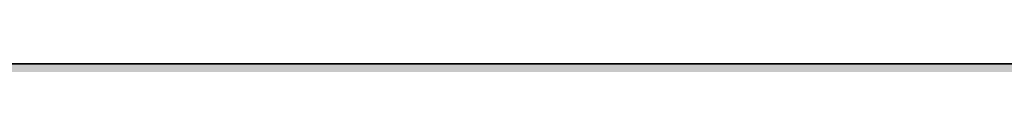
# Model space of a CAD drawing. Units: inches. Extents: x 2091 to 2899, y 967 to 2217.
# Tile 97 of 256: x 2251.8124 to 2252.3817, y 1099.9191 to 1099.9191. Entities that reach past the tile are written whole.
import ezdxf

# ---------------------------------------------------------------- set-up
doc = ezdxf.new("R2010")
doc.units = ezdxf.units.IN
doc.layers.add('A-WALL-PATT', color=141, linetype='Continuous', lineweight=13, true_color=0xadddf7)
doc.layers.add('L-SITE-WALL', color=7, linetype='Continuous', lineweight=35)

msp = doc.modelspace()

# ---------------------------------------------------------------- hatches: boundary and pattern name
at = {"layer": 'A-WALL-PATT'}
h = msp.add_hatch(color=256, dxfattribs=at)
h.dxf.hatch_style = 1
h.paths.add_polyline_path([(2212.1436, 1941.41906), (2387.6436, 1941.41906), (2387.6436, 1824.41906), (2392.1436, 1824.41906), (2392.1436, 1941.41906), (2609.6436, 1941.41906), (2609.6436, 1825.91906), (2614.1436, 1825.91906), (2614.1436, 1941.41906), (2794.1436, 1941.41906), (2794.1436, 1928.76217), (2803.1436, 1928.76217), (2803.1436, 2050.91906), (2203.1436, 2050.91906), (2203.1436, 1900.75786), (2212.1436, 1900.75786)])
h.paths.add_polyline_path([(2212.1436, 1945.91906), (2212.1436, 2041.91906), (2794.1436, 2041.91906), (2794.1436, 1945.91906), (2402.24824, 1945.91906), (2401.10243, 1945.77583), (2398.70243, 1945.77583)], flags=16)
h.paths.add_polyline_path([(2230.22986, 1948.06279), (2227.34986, 1949.50279), (2225.90986, 1951.90279), (2223.98986, 1952.86279), (2223.02986, 1955.26279), (2222.06986, 1959.58279), (2222.06986, 1963.42279), (2223.02986, 1965.66279), (2223.98986, 1965.34279), (2225.58591, 1963.86075), (2226.91153, 1964.95726), (2226.94886, 1965.93879), (2227.77832, 1966.95214), (2228.19992, 1968.8787), (2230.70986, 1964.86279), (2233.58986, 1966.30279), (2233.60731, 1966.33187), (2233.77266, 1964.9382), (2234.6338, 1963.67647), (2235.02986, 1963.90279), (2236.28203, 1965.57236), (2235.98986, 1962.94279), (2237.95451, 1957.54), (2238.38986, 1957.90279), (2239.21586, 1960.30579), (2238.65457, 1966.38496), (2238.69279, 1966.43807), (2238.84058, 1967.49971), (2238.78029, 1967.68749), (2238.88054, 1967.78676), (2238.66686, 1966.25179), (2239.21586, 1960.30579), (2238.38986, 1957.90279), (2236.94986, 1956.70279), (2234.54986, 1949.98279)], flags=0)
h.paths.add_polyline_path([(2278.01197, 1948.06279), (2276.49643, 1947.87335), (2275.84983, 1947.68861), (2274.65197, 1947.10279)], flags=0)
h.paths.add_polyline_path([(2269.85197, 1955.74279), (2268.27618, 1956.62933), (2270.8673, 1956.3484), (2269.37197, 1958.14279), (2268.71496, 1959.19233), (2270.56983, 1958.72861), (2268.58073, 1961.90609), (2270.81197, 1960.89188), (2270.81197, 1963.42279), (2271.39331, 1964.77926), (2270.29176, 1966.1562), (2271.77197, 1965.66279), (2272.14139, 1966.52476), (2273.92983, 1965.92861), (2275.63039, 1968.0543), (2276.33194, 1966.72186), (2276.52043, 1966.95214), (2276.94203, 1968.8787), (2277.73429, 1967.61108), (2278.13989, 1969.46452), (2279.65912, 1967.03374), (2280.41197, 1966.78279), (2280.9493, 1967.58879), (2281.60983, 1967.36861), (2282.13327, 1968.15376), (2282.34924, 1966.33344), (2282.34985, 1966.33259), (2283.40755, 1968.09542), (2283.71263, 1965.52402), (2284.32022, 1964.63379), (2284.51181, 1964.88924), (2284.23497, 1965.70479), (2284.50047, 1967.31896), (2284.90794, 1965.41742), (2285.39631, 1966.06858), (2285.43283, 1966.29061), (2285.47334, 1966.17128), (2286.35392, 1967.34539), (2286.22201, 1966.15817), (2287.66349, 1968.08015), (2287.71397, 1968.44279), (2288.4816, 1969.01668), (2288.57399, 1968.7289), (2288.91746, 1969.06904), (2288.60683, 1966.83761), (2288.92873, 1963.35131), (2288.93497, 1963.35679), (2288.92973, 1963.34042), (2289.01528, 1962.41387), (2290.11122, 1963.87513), (2290.13283, 1963.94261), (2290.21767, 1964.01706), (2290.11122, 1963.87513), (2289.15583, 1960.89161), (2288.59404, 1959.25723), (2288.57197, 1959.10279), (2289.53197, 1960.54279), (2290.01197, 1962.46279), (2290.19184, 1962.64266), (2289.76983, 1959.68861), (2286.88983, 1957.28861), (2284.48983, 1950.56861), (2283.31466, 1950.04631), (2283.29197, 1949.98279), (2280.29006, 1948.64861), (2281.12983, 1948.64861), (2282.56983, 1948.16861), (2283.20473, 1948.06279), (2278.97197, 1948.06279), (2276.09197, 1949.50279), (2274.65197, 1951.90279), (2272.73197, 1952.86279)], flags=0)
h.paths.add_polyline_path([(2271.15887, 1958.02177), (2272.96983, 1955.84861), (2272.00983, 1960.16861), (2272.00983, 1964.00861), (2272.62443, 1965.44266), (2274.32802, 1963.86075), (2275.65365, 1964.95726), (2275.63774, 1964.53909), (2277.41223, 1966.00689), (2277.03297, 1965.15679), (2276.82992, 1964.9756), (2276.76601, 1963.29501), (2277.44964, 1962.66022), (2279.45197, 1964.86279), (2282.33197, 1966.30279), (2283.52983, 1966.88861), (2283.29451, 1966.77095), (2283.91299, 1963.8847), (2284.89925, 1964.44827), (2284.73197, 1962.94279), (2286.69662, 1957.54), (2287.13197, 1957.90279), (2287.54191, 1959.09539), (2287.7794, 1958.44231), (2285.68274, 1956.6951), (2285.8765, 1959.79534), (2284.73197, 1962.94279), (2284.89925, 1964.44827), (2283.91299, 1963.8847), (2284.22383, 1962.43412), (2283.42436, 1963.60548), (2281.60983, 1962.56861), (2281.12983, 1960.16861), (2282.08983, 1956.32861), (2283.04983, 1952.96861), (2282.56983, 1950.56861), (2280.16983, 1948.64861), (2279.88332, 1948.79187), (2278.97197, 1948.06279), (2278.97197, 1949.02279), (2278.67231, 1949.39737), (2277.28983, 1950.08861), (2275.84983, 1952.48861), (2273.92983, 1953.44861), (2272.48983, 1954.88861), (2271.92165, 1954.88861), (2271.77197, 1955.26279)], flags=0)
h.paths.add_polyline_path([(2311.99415, 1955.74279), (2312.06272, 1955.67422), (2312.0551, 1955.7085)], flags=0)
h.paths.add_polyline_path([(2331.95615, 1963.95179), (2333.39615, 1965.39179), (2331.07715, 1963.35679), (2330.9986, 1963.11152)], flags=0)
h.paths.add_polyline_path([(2310.55415, 1954.30279), (2307.03981, 1956.27994), (2310.7629, 1955.87628), (2312.47415, 1953.82279), (2313.43415, 1951.42279), (2315.35415, 1950.46279), (2316.79415, 1948.06279), (2317.46615, 1947.72679), (2319.36869, 1947.96461), (2317.75415, 1949.98279), (2317.56953, 1950.61048), (2316.79415, 1951.90279), (2314.87415, 1952.86279), (2313.91415, 1955.26279), (2311.51415, 1958.14279), (2309.37549, 1961.55917), (2311.51415, 1960.33708), (2311.51415, 1961.98279), (2310.60467, 1963.11963), (2311.72661, 1962.47853), (2312.41833, 1964.09256), (2312.25596, 1964.29552), (2313.19415, 1963.98279), (2313.91415, 1965.66279), (2314.64678, 1965.41858), (2315.35415, 1966.30279), (2316.79415, 1967.74279), (2316.15744, 1966.9469), (2317.03411, 1965.28186), (2317.2226, 1965.51214), (2317.77705, 1968.04577), (2318.47411, 1966.72186), (2318.6626, 1966.95214), (2319.0842, 1968.8787), (2321.20705, 1965.48215), (2322.16142, 1966.9137), (2322.55415, 1966.78279), (2322.78599, 1967.13056), (2322.88165, 1966.32429), (2323.31204, 1965.72174), (2323.65129, 1965.89136), (2324.3965, 1967.13338), (2324.65694, 1964.9382), (2324.97199, 1964.47661), (2325.38728, 1967.0015), (2325.94081, 1964.41835), (2327.22893, 1966.13584), (2327.16632, 1965.57236), (2328.05914, 1966.76278), (2328.22458, 1966.24749), (2329.66797, 1967.67691), (2329.66458, 1967.68749), (2329.76482, 1967.78676), (2329.55115, 1966.25179), (2330.10015, 1960.30579), (2329.33281, 1958.07347), (2329.31306, 1957.93523), (2329.63415, 1958.20279), (2330.23415, 1959.10279), (2330.71415, 1961.02279), (2331.03415, 1961.34279), (2330.71415, 1959.10279), (2329.63415, 1958.20279), (2329.27415, 1957.66279), (2327.71211, 1956.3611), (2325.43415, 1949.98279), (2324.33377, 1949.49374), (2323.99415, 1948.54279), (2319.67415, 1946.62279), (2316.79415, 1948.06279), (2315.35415, 1950.46279), (2313.43415, 1951.42279)], flags=0)
h.paths.add_polyline_path([(2321.33568, 1947.95202), (2321.11415, 1948.06279), (2321.11415, 1949.02279), (2319.19415, 1951.42279), (2316.79415, 1959.58279), (2316.66324, 1959.58279), (2315.35415, 1958.14279), (2314.39415, 1958.14279), (2313.1483, 1958.70908), (2312.95415, 1959.58279), (2312.95415, 1960.89188), (2315.83415, 1959.58279), (2316.66324, 1959.58279), (2317.31471, 1960.29941), (2315.0302, 1962.42075), (2316.35582, 1963.51726), (2316.37234, 1963.95162), (2316.4702, 1963.86075), (2317.79582, 1964.95726), (2317.75522, 1963.88969), (2319.17515, 1965.15679), (2319.49841, 1965.88137), (2321.11415, 1965.34279), (2323.23589, 1962.37236), (2325.68635, 1963.77262), (2325.54279, 1962.48058), (2325.19878, 1963.49401), (2324.47851, 1963.08243), (2324.92601, 1960.99412), (2324.07809, 1962.23647), (2322.41479, 1961.28602), (2322.07415, 1959.58279), (2323.03415, 1955.74279), (2323.99415, 1952.38279), (2323.51415, 1949.98279), (2322.14272, 1948.88565), (2322.07415, 1948.54279)], flags=0)
h.paths.add_polyline_path([(2320.20748, 1963.33746), (2320.15415, 1963.42279), (2320.39415, 1963.54279)], flags=0)
h.paths.add_polyline_path([(2353.85053, 1965.8105), (2354.03053, 1965.7505), (2354.33053, 1966.4505), (2354.33053, 1966.9305)], flags=0)
h.paths.add_polyline_path([(2359.02058, 1969.02641), (2359.09838, 1968.90193), (2359.23353, 1969.5195), (2359.23353, 1969.9995)], flags=0)
h.paths.add_polyline_path([(2358.25669, 1966.68167), (2357.9836, 1966.34803), (2358.21127, 1966.14617), (2358.41049, 1966.38957)], flags=0)
h.paths.add_polyline_path([(2357.76847, 1966.05878), (2357.7322, 1965.10497), (2357.75105, 1965.12056), (2357.76953, 1965.6065), (2357.76953, 1966.05784)], flags=0)
h.paths.add_polyline_path([(2359.11153, 1965.3045), (2359.11153, 1964.8245), (2359.84453, 1966.4675), (2359.84453, 1966.9475)], flags=0)
h.paths.add_polyline_path([(2360.22368, 1966.62145), (2360.69853, 1969.3625), (2360.69853, 1969.8425), (2360.21053, 1967.0255), (2360.21053, 1966.6425)], flags=0)
h.paths.add_polyline_path([(2363.45053, 1967.8905), (2363.45053, 1968.3705), (2362.49053, 1966.9305), (2362.65604, 1966.69878)], flags=0)
h.paths.add_polyline_path([(2364.47552, 1966.07883), (2365.85053, 1968.3705), (2365.85053, 1968.8505), (2364.42798, 1966.47958)], flags=0)
h.paths.add_polyline_path([(2366.31353, 1965.8525), (2366.36671, 1965.69583), (2366.80253, 1968.3455), (2366.80253, 1968.8255)], flags=0)
h.paths.add_polyline_path([(2367.16531, 1965.80354), (2367.29053, 1966.9305), (2367.29053, 1967.4105), (2367.1027, 1965.72007)], flags=0)
h.paths.add_polyline_path([(2370.03653, 1959.9735), (2371.01353, 1963.0245), (2371.01353, 1963.5045), (2370.03653, 1960.4535)], flags=0)
h.paths.add_polyline_path([(2371.61053, 1960.2105), (2372.57053, 1961.6505), (2372.57053, 1962.1305), (2371.80253, 1960.9785)], flags=0)
h.paths.add_polyline_path([(2350.87367, 1956.00509), (2351.93053, 1955.8905), (2354.49053, 1953.3305), (2353.85053, 1954.9305), (2351.45053, 1957.8105), (2347.93553, 1963.4255), (2347.93553, 1963.9055), (2351.45053, 1958.2905), (2353.70507, 1955.58505), (2352.89053, 1959.2505), (2352.89053, 1959.7305), (2352.89053, 1961.92479), (2356.73053, 1959.7305), (2358.45447, 1961.62684), (2354.81053, 1965.0105), (2355.03086, 1965.28591), (2358.69109, 1961.88712), (2361.53053, 1965.0105), (2364.3765, 1966.43348), (2364.52439, 1965.18691), (2365.45447, 1963.82418), (2365.88107, 1964.06795), (2365.37053, 1966.4505), (2365.37053, 1966.9305), (2366.81053, 1960.2105), (2366.81053, 1959.7305), (2366.38871, 1952.98141), (2367.77053, 1956.8505), (2368.64123, 1957.57608), (2366.81053, 1962.6105), (2366.81053, 1963.0905), (2368.77518, 1957.68771), (2369.21053, 1958.0505), (2370.00159, 1960.35187), (2369.47523, 1966.05267), (2369.51346, 1966.10578), (2369.51417, 1966.11091), (2369.47523, 1966.53267), (2369.51346, 1966.58578), (2369.61463, 1967.31259), (2369.18253, 1968.6585), (2369.18253, 1969.1385), (2369.60096, 1967.83519), (2369.7012, 1967.93447), (2369.71795, 1968.05474), (2370.14518, 1968.37414), (2369.77871, 1968.01122), (2369.7012, 1967.45447), (2370.46816, 1968.214), (2369.67494, 1967.26577), (2369.51417, 1966.11091), (2370.03653, 1960.4535), (2370.03653, 1959.9735), (2369.44176, 1958.24319), (2370.65053, 1959.2505), (2371.04582, 1962.01756), (2371.13053, 1962.1305), (2370.65053, 1958.7705), (2367.77053, 1956.3705), (2365.37053, 1949.6505), (2362.0791, 1948.18764), (2363.45053, 1947.7305), (2361.05053, 1947.7305), (2360.09053, 1947.7305), (2357.10386, 1947.35717), (2360.09053, 1948.2105), (2358.17053, 1949.1705), (2356.73053, 1951.5705), (2354.81053, 1952.5305), (2351.93053, 1955.4105)], flags=0)
h.paths.add_polyline_path([(2361.05053, 1948.6905), (2359.13053, 1951.0905), (2356.73053, 1959.2505), (2355.77053, 1959.2505), (2352.89053, 1960.55959), (2352.89053, 1961.44479), (2355.89053, 1959.7305), (2356.73053, 1959.7305), (2356.83719, 1959.36783), (2361.53053, 1964.5305), (2363.24842, 1965.38945), (2364.92531, 1963.0418), (2362.49053, 1961.6505), (2362.06386, 1959.51717), (2362.97053, 1955.8905), (2363.93053, 1952.5305), (2363.93053, 1952.0505), (2363.45053, 1949.6505), (2361.05053, 1947.7305)], flags=0)
h.paths.add_polyline_path([(2359.13053, 1951.5705), (2359.29053, 1951.3705), (2361.05053, 1954.4505), (2361.05053, 1954.9305)], flags=0)
h.paths.add_polyline_path([(2357.21953, 1966.5455), (2356.79253, 1968.8145), (2356.79253, 1969.2945), (2357.21953, 1967.0255)], flags=0)
h.paths.add_polyline_path([(2361.05053, 1954.4505), (2361.53053, 1958.7705), (2361.53053, 1959.2505), (2361.05053, 1954.9305)], flags=0)
h.paths.add_polyline_path([(2402.54829, 1948.48608), (2402.30243, 1948.41583), (2402.59043, 1948.41583)], flags=0)
h.paths.add_polyline_path([(2394.14243, 1956.09583), (2395.68505, 1954.55321), (2396.7205, 1953.97068), (2396.06243, 1955.61583), (2395.24138, 1956.6011), (2395.8789, 1956.44171), (2395.10243, 1959.93583), (2395.10243, 1963.77583), (2396.06243, 1966.01583), (2397.02243, 1965.69583), (2398.61848, 1964.21379), (2399.94411, 1965.3103), (2399.98143, 1966.29183), (2400.81089, 1967.30518), (2401.23249, 1969.23174), (2403.53795, 1965.54301), (2403.94198, 1967.38932), (2404.70243, 1967.13583), (2405.46033, 1966.07478), (2406.62243, 1966.65583), (2406.63988, 1966.68491), (2406.80523, 1965.29124), (2406.92569, 1965.11475), (2407.34243, 1964.97583), (2407.87433, 1965.77367), (2408.1691, 1964.39805), (2409.31461, 1965.9254), (2409.21746, 1965.05105), (2409.44523, 1963.13124), (2410.30637, 1961.86951), (2410.70243, 1962.09583), (2411.44227, 1963.08228), (2411.16543, 1963.89783), (2411.61643, 1966.63976), (2411.72536, 1966.79111), (2411.87315, 1967.85275), (2411.81286, 1968.04053), (2411.91311, 1968.1398), (2411.69943, 1966.60483), (2412.24843, 1960.65883), (2413.22543, 1963.70983), (2414.3779, 1964.72116), (2414.51315, 1965.69275), (2414.45286, 1965.88053), (2414.55311, 1965.9798), (2414.3779, 1964.72116), (2414.51982, 1964.8457), (2414.36536, 1964.63111), (2414.33943, 1964.44483), (2414.88843, 1958.49883), (2414.06243, 1956.09583), (2412.62243, 1954.89583), (2410.17137, 1948.03285), (2410.01672, 1948.0844), (2405.90243, 1946.25583), (2405.90243, 1947.21583), (2405.20425, 1948.08856), (2404.22243, 1948.41583), (2403.26243, 1948.41583), (2400.38243, 1949.85583), (2399.66243, 1951.05583), (2397.98243, 1952.73583), (2397.02243, 1953.21583), (2395.68505, 1954.55321), (2392.65678, 1956.25691)], flags=0)
h.paths.add_polyline_path([(2409.08565, 1964.40744), (2409.13036, 1964.27572), (2409.26243, 1964.49583)], flags=0)
h.paths.add_polyline_path([(2397.74243, 1961.61583), (2398.70243, 1963.85583), (2399.66243, 1963.53583), (2401.42656, 1965.74099), (2401.79142, 1966.5588), (2402.07143, 1965.07083), (2402.83551, 1964.39337), (2403.2624, 1964.9149), (2403.33812, 1964.77109), (2402.61552, 1963.97622), (2402.49861, 1960.90224), (2403.543, 1959.93245), (2404.4132, 1960.88968), (2404.70243, 1962.33583), (2407.91635, 1964.17235), (2409.52021, 1961.92694), (2410.98708, 1957.89304), (2411.42243, 1958.25583), (2412.04796, 1960.07562), (2412.41034, 1959.07909), (2411.67562, 1958.46682), (2411.66243, 1958.25583), (2411.62607, 1958.42553), (2409.98243, 1957.05583), (2407.58243, 1950.33583), (2403.26243, 1948.41583), (2403.26243, 1949.37583), (2401.34243, 1951.77583), (2399.41651, 1958.32398), (2397.74243, 1959.08492), (2397.74243, 1959.97012), (2397.10243, 1960.33583), (2397.74243, 1960.04492)], flags=0)
h.paths.add_polyline_path([(2405.90243, 1952.97583), (2405.95043, 1953.40783), (2406.01672, 1953.17583)], flags=0)
h.paths.add_polyline_path([(2449.81778, 1967.11401), (2449.75232, 1967.13583), (2449.7937, 1967.0779)], flags=0)
h.paths.add_polyline_path([(2451.6977, 1966.61812), (2451.74089, 1966.69012), (2451.69205, 1966.6657)], flags=0)
h.paths.add_polyline_path([(2454.34363, 1965.73757), (2455.75232, 1967.61583), (2455.99232, 1968.09583), (2454.3645, 1965.9254)], flags=0)
h.paths.add_polyline_path([(2457.54732, 1968.86383), (2457.78732, 1969.34383), (2457.05432, 1968.79583), (2457.00762, 1968.46034)], flags=0)
h.paths.add_polyline_path([(2456.92178, 1967.85666), (2456.80224, 1968.22902), (2456.723, 1967.6598)], flags=0)
h.paths.add_polyline_path([(2457.30232, 1967.37683), (2457.54232, 1967.85683), (2456.81032, 1966.83983), (2456.74052, 1966.70022), (2456.74902, 1966.60811)], flags=0)
h.paths.add_polyline_path([(2458.27532, 1963.70983), (2458.15534, 1963.33515), (2460.35432, 1965.26483), (2460.59432, 1965.74483)], flags=0)
h.paths.add_polyline_path([(2458.39232, 1962.81583), (2458.36409, 1962.61819), (2459.59232, 1964.25583), (2459.83232, 1964.73583)], flags=0)
h.paths.add_polyline_path([(2459.35232, 1962.81583), (2459.27232, 1962.49583), (2460.07232, 1963.29583), (2460.31232, 1963.77583)], flags=0)
h.paths.add_polyline_path([(2458.68032, 1960.60783), (2458.63232, 1960.41583), (2459.59232, 1961.85583), (2459.83232, 1962.33583)], flags=0)
h.paths.add_polyline_path([(2437.83817, 1956.24265), (2439.19232, 1956.09583), (2441.35232, 1953.93583), (2440.87232, 1955.13583), (2438.47232, 1958.01583), (2438.07156, 1958.65602), (2438.71232, 1958.49583), (2440.6396, 1956.18311), (2439.91232, 1959.45583), (2439.91232, 1963.29583), (2441.35232, 1966.65583), (2441.59232, 1967.13583), (2441.11232, 1966.01583), (2442.07232, 1965.69583), (2443.98899, 1968.09167), (2444.24132, 1966.75083), (2444.9168, 1966.15192), (2445.67657, 1967.08014), (2446.25532, 1969.72483), (2446.49532, 1970.20483), (2446.28238, 1969.23174), (2447.36267, 1967.50327), (2447.72032, 1969.56783), (2447.96032, 1970.04783), (2447.48548, 1967.30678), (2448.79232, 1965.21583), (2448.47232, 1964.86383), (2448.55232, 1964.73583), (2451.45205, 1966.1857), (2451.61512, 1964.81124), (2452.30792, 1963.79617), (2453.23451, 1964.32565), (2454.07232, 1960.41583), (2453.62869, 1953.31765), (2454.79232, 1956.57583), (2455.03232, 1957.05583), (2455.71884, 1957.62793), (2453.83232, 1962.81583), (2453.94097, 1963.79362), (2453.33532, 1965.57783), (2453.82432, 1968.55083), (2454.06432, 1969.03083), (2453.57532, 1966.05783), (2454.04033, 1964.68792), (2453.83232, 1962.81583), (2455.71884, 1957.62793), (2456.36721, 1958.16824), (2457.05832, 1960.17883), (2457.29832, 1960.65883), (2456.47232, 1958.25583), (2457.71773, 1959.29367), (2457.67232, 1958.97583), (2454.88995, 1956.65719), (2453.61414, 1953.08492), (2453.59232, 1952.73583), (2453.35232, 1952.25583), (2453.3596, 1952.3722), (2452.63232, 1950.33583), (2452.39232, 1949.85583), (2449.20375, 1948.43869), (2450.71232, 1947.93583), (2448.07232, 1947.93583), (2447.11232, 1947.93583), (2444.55232, 1947.61583), (2447.1996, 1948.3722), (2445.19232, 1949.37583), (2443.75232, 1951.77583), (2441.83232, 1952.73583), (2438.95232, 1955.61583)], flags=0)
h.paths.add_polyline_path([(2443.99232, 1959.93583), (2444.04032, 1959.77263), (2444.12155, 1959.86199)], flags=0)
h.paths.add_polyline_path([(2442.91232, 1959.93583), (2443.03232, 1959.93583), (2442.44566, 1960.2025)], flags=0)
h.paths.add_polyline_path([(2444.98294, 1965.01968), (2445.27932, 1965.26483), (2445.51932, 1965.74483), (2444.994, 1965.3103)], flags=0)
h.paths.add_polyline_path([(2446.13332, 1965.02983), (2446.33037, 1965.4715), (2444.97032, 1964.25783), (2444.73032, 1963.77783)], flags=0)
h.paths.add_polyline_path([(2442.79232, 1959.45583), (2443.75232, 1959.45583), (2446.15232, 1951.29583), (2446.41232, 1951.75083), (2446.39232, 1951.77583), (2448.0806, 1954.73032), (2448.55232, 1958.97583), (2441.83232, 1965.21583), (2442.15495, 1965.61911), (2448.79232, 1959.45583), (2448.31232, 1955.13583), (2448.07232, 1954.65583), (2446.41232, 1951.75083), (2448.31232, 1949.37583), (2448.31232, 1948.41583), (2450.54089, 1950.19869), (2450.95232, 1952.25583), (2449.99232, 1955.61583), (2449.03232, 1959.45583), (2449.51232, 1961.85583), (2449.75232, 1962.33583), (2449.6749, 1961.94874), (2452.99451, 1963.84565), (2453.06441, 1963.51941), (2452.88461, 1963.78285), (2449.6749, 1961.94874), (2449.27232, 1959.93583), (2450.23232, 1956.09583), (2451.19232, 1952.73583), (2450.71232, 1950.33583), (2450.47232, 1949.85583), (2448.07232, 1947.93583), (2448.07232, 1948.53583), (2445.43232, 1949.85583), (2443.99232, 1952.25583), (2442.07232, 1953.21583), (2441.11232, 1955.61583), (2440.15232, 1959.93583), (2440.15232, 1960.65583)], flags=0)
h.paths.add_polyline_path([(2456.69232, 1966.98583), (2457.60832, 1968.08083), (2457.84832, 1968.56083), (2456.93232, 1967.46583)], flags=0)
h.paths.add_polyline_path([(2489.89657, 1966.58024), (2489.94295, 1966.18935), (2490.74749, 1967.53025), (2491.31912, 1968.95116)], flags=0)
h.paths.add_polyline_path([(2473.56247, 1956.40713), (2477.13998, 1956.01926), (2476.95533, 1956.24083), (2475.10805, 1957.28011), (2476.34749, 1956.97025), (2475.1869, 1958.82422), (2476.91912, 1958.39116), (2475.41164, 1960.79927), (2477.78749, 1959.71934), (2477.78749, 1962.25025), (2477.6374, 1962.43786), (2477.82255, 1962.33206), (2478.35912, 1963.58406), (2478.35912, 1963.67116), (2477.32435, 1964.96463), (2478.71483, 1964.50114), (2479.31912, 1965.91116), (2480.27912, 1965.59116), (2481.78397, 1967.47221), (2482.11649, 1965.70525), (2482.88056, 1965.02778), (2483.20931, 1965.42941), (2483.22017, 1965.71509), (2483.07594, 1965.98902), (2483.71176, 1966.76581), (2484.13049, 1968.67925), (2484.70212, 1970.10016), (2484.48918, 1969.12707), (2486.5029, 1965.90511), (2487.38749, 1965.61025), (2488.15342, 1966.75914), (2488.71702, 1965.97011), (2489.20009, 1966.21164), (2489.33067, 1965.11099), (2490.3939, 1963.62246), (2490.66077, 1963.77496), (2490.49391, 1964.55364), (2490.92306, 1963.92484), (2491.31912, 1964.15116), (2491.33339, 1964.17018), (2491.21049, 1964.53225), (2491.28176, 1964.96554), (2491.42579, 1964.29338), (2494.07648, 1967.82763), (2494.49792, 1966.51494), (2494.59817, 1966.61422), (2494.68949, 1967.27025), (2495.10675, 1967.5822), (2495.12984, 1967.74807), (2495.06955, 1967.93585), (2495.1698, 1968.03513), (2495.03178, 1967.04363), (2495.75382, 1967.75868), (2494.98205, 1966.68644), (2494.95612, 1966.50016), (2495.47902, 1960.83685), (2495.91049, 1962.18425), (2496.48212, 1963.60516), (2496.07269, 1962.32659), (2496.7689, 1962.93754), (2496.59912, 1962.71116), (2496.11912, 1959.35116), (2496.73287, 1960.27179), (2496.98749, 1961.29025), (2497.55912, 1962.71116), (2497.07912, 1960.79116), (2496.50749, 1959.37025), (2495.54749, 1957.93025), (2492.75884, 1955.60638), (2490.83912, 1950.23116), (2490.26749, 1948.81025), (2485.94749, 1946.89025), (2483.06749, 1948.33025), (2481.62749, 1950.73025), (2479.70749, 1951.69025), (2476.82749, 1954.57025)], flags=0)
h.paths.add_polyline_path([(2485.57697, 1948.31339), (2485.55912, 1948.31116), (2485.57876, 1948.31116)], flags=0)
h.paths.add_polyline_path([(2478.64506, 1954.55116), (2478.10904, 1956.96326), (2479.31912, 1955.51116), (2480.27912, 1953.11116), (2482.19912, 1952.15116), (2483.63912, 1949.75116), (2486.51912, 1948.31116), (2486.51912, 1949.27116), (2484.73931, 1951.49593), (2484.02749, 1950.25025), (2481.62749, 1958.41025), (2482.37515, 1959.23267), (2482.19912, 1959.83116), (2483.19757, 1960.92946), (2479.70749, 1964.17025), (2480.60336, 1965.29008), (2481.87517, 1964.10911), (2482.66639, 1964.76358), (2482.61536, 1963.4218), (2482.9892, 1963.07466), (2484.00849, 1963.98425), (2484.68361, 1965.49751), (2484.58012, 1965.40516), (2485.35727, 1967.14711), (2485.12065, 1965.7812), (2486.42749, 1963.69025), (2488.14538, 1964.5492), (2489.82227, 1962.20155), (2490.74749, 1962.73025), (2491.99966, 1964.39981), (2492.07605, 1965.08726), (2492.21289, 1964.68412), (2492.48537, 1965.04743), (2492.27912, 1963.19116), (2494.24377, 1957.78837), (2494.5625, 1958.05398), (2494.93349, 1959.13325), (2495.50512, 1960.55416), (2494.67912, 1958.15116), (2494.10749, 1956.73025), (2494.5625, 1958.05398), (2493.40854, 1957.09235), (2491.70749, 1961.77025), (2491.99966, 1964.39981), (2490.74749, 1962.73025), (2487.71203, 1960.9957), (2487.47912, 1959.83116), (2488.43912, 1955.99116), (2489.39912, 1952.63116), (2488.91912, 1950.23116), (2488.57692, 1949.9574), (2488.34749, 1948.81025), (2487.65172, 1948.25363), (2487.47912, 1948.31116), (2486.51912, 1948.31116), (2483.63912, 1949.75116), (2482.19912, 1952.15116), (2480.27912, 1953.11116), (2478.83912, 1954.55116)], flags=0)
h.paths.add_polyline_path([(2526.64825, 1966.98752), (2526.51734, 1967.03116), (2526.6001, 1966.9153)], flags=0)
h.paths.add_polyline_path([(2528.47064, 1966.44666), (2528.57449, 1966.61973), (2528.45707, 1966.56102)], flags=0)
h.paths.add_polyline_path([(2534.13334, 1967.49616), (2534.15669, 1967.54285), (2534.05984, 1967.4083)], flags=0)
h.paths.add_polyline_path([(2536.16192, 1964.0506), (2535.15734, 1962.71116), (2535.10087, 1962.31587), (2536.11734, 1963.67116), (2536.42053, 1964.27754)], flags=0)
h.paths.add_polyline_path([(2535.15734, 1959.83116), (2536.11734, 1961.27116), (2536.59734, 1962.23116), (2535.25334, 1960.21516)], flags=0)
h.paths.add_polyline_path([(2513.24904, 1956.2848), (2516.22118, 1955.96256), (2514.99734, 1957.43116), (2514.19582, 1958.71154), (2515.47734, 1958.39116), (2516.93189, 1956.64571), (2516.43734, 1958.87116), (2516.43734, 1962.71116), (2516.87269, 1963.72697), (2515.34643, 1965.6348), (2517.39734, 1964.95116), (2517.87734, 1966.07116), (2518.35734, 1967.03116), (2517.87734, 1965.91116), (2518.83734, 1965.59116), (2520.48659, 1967.65272), (2520.76634, 1966.16616), (2521.53042, 1965.48869), (2521.78144, 1965.79537), (2521.80091, 1966.30727), (2521.4778, 1966.92094), (2521.24634, 1967.12616), (2521.1777, 1967.49091), (2521.4778, 1966.92094), (2522.01042, 1966.44869), (2522.25739, 1966.75042), (2522.78034, 1969.14016), (2523.26034, 1970.10016), (2523.0474, 1969.12707), (2524.67313, 1966.5259), (2526.03734, 1966.07116), (2526.79524, 1965.01011), (2527.97707, 1965.60102), (2528.14014, 1964.22657), (2528.66459, 1963.45816), (2529.38862, 1963.87189), (2529.32967, 1964.14699), (2529.48128, 1963.92484), (2529.87734, 1964.15116), (2529.98401, 1964.29338), (2529.78905, 1965.20318), (2530.0624, 1964.3979), (2532.80248, 1968.05135), (2533.14777, 1966.97585), (2533.24802, 1967.07513), (2533.33934, 1967.73116), (2533.67285, 1967.98049), (2533.72802, 1968.03513), (2533.51434, 1966.50016), (2534.02472, 1960.9725), (2534.56034, 1962.64516), (2535.04034, 1963.60516), (2534.06334, 1960.55416), (2533.23734, 1958.15116), (2534.28815, 1959.02684), (2534.19734, 1958.39116), (2531.5126, 1956.15387), (2529.39734, 1950.23116), (2528.91734, 1949.27116), (2526.44877, 1948.17402), (2527.47734, 1947.83116), (2530.35734, 1947.35116), (2524.59734, 1947.35116), (2521.71734, 1948.79116), (2520.27734, 1951.19116), (2518.35734, 1952.15116), (2515.47734, 1955.03116)], flags=0)
h.paths.add_polyline_path([(2523.93476, 1967.19031), (2523.61951, 1966.48369), (2523.7705, 1966.24211)], flags=0)
h.paths.add_polyline_path([(2518.83734, 1953.11116), (2517.87734, 1955.51116), (2516.88498, 1959.97678), (2516.91734, 1959.96207), (2516.91734, 1962.02545), (2520.75734, 1959.83116), (2522.02495, 1961.22553), (2518.35734, 1964.63116), (2519.00259, 1965.43772), (2520.43339, 1964.10911), (2521.30112, 1964.82687), (2521.24516, 1963.35533), (2525.63831, 1959.27598), (2526.03734, 1961.27116), (2529.39734, 1963.19116), (2530.64952, 1964.86073), (2530.66472, 1964.99755), (2530.69196, 1964.91731), (2531.08778, 1965.44507), (2530.94599, 1964.16894), (2530.69196, 1964.91731), (2529.39734, 1963.19116), (2526.3625, 1961.45697), (2526.03734, 1959.83116), (2526.99734, 1955.99116), (2527.95734, 1952.63116), (2527.47734, 1950.23116), (2527.13449, 1949.95687), (2526.97393, 1949.15409), (2526.69734, 1949.03116), (2524.59734, 1947.35116), (2524.59734, 1948.31116), (2524.27734, 1948.71116), (2522.19734, 1949.75116), (2520.75734, 1952.15116)], flags=0)
h.paths.add_polyline_path([(2520.27734, 1958.87116), (2520.85334, 1959.50476), (2523.15734, 1951.67116), (2524.61389, 1954.22013), (2524.59734, 1954.07116), (2522.67734, 1950.71116)], flags=0)
h.paths.add_polyline_path([(2559.37091, 1966.31116), (2559.39841, 1966.32491), (2559.40194, 1966.3453)], flags=0)
h.paths.add_polyline_path([(2549.77091, 1957.19116), (2552.65091, 1954.31116), (2552.13399, 1955.60347), (2550.61091, 1957.43116), (2547.09591, 1963.04616), (2545.77591, 1965.20616), (2549.29091, 1959.59116), (2551.69091, 1956.71116), (2550.79293, 1960.75206), (2550.73091, 1960.78025), (2550.73091, 1964.87116), (2551.69091, 1967.11116), (2552.65091, 1966.79116), (2554.24696, 1965.30911), (2555.03425, 1965.96034), (2555.58167, 1966.64461), (2555.60991, 1967.38716), (2556.43937, 1968.40051), (2556.86097, 1970.32707), (2559.37091, 1966.31116), (2560.69091, 1964.15116), (2562.40881, 1965.01011), (2561.65091, 1966.07116), (2560.33091, 1968.23116), (2561.7585, 1966.23254), (2562.34721, 1967.11561), (2562.43371, 1966.38657), (2563.1278, 1965.3696), (2563.57091, 1965.59116), (2563.58836, 1965.62024), (2563.36254, 1967.52354), (2563.72249, 1965.84379), (2565.06, 1968.07298), (2564.73286, 1965.12872), (2565.11758, 1963.33338), (2567.44462, 1966.43611), (2567.31561, 1967.83333), (2567.35384, 1967.88644), (2567.50163, 1968.94807), (2567.44134, 1969.13585), (2567.54159, 1969.23513), (2567.32791, 1967.70016), (2567.87691, 1961.75416), (2568.74669, 1964.47033), (2568.63561, 1965.67333), (2568.67384, 1965.72644), (2568.82163, 1966.78807), (2568.76134, 1966.97585), (2568.86159, 1967.07513), (2568.64791, 1965.54016), (2568.72613, 1964.69303), (2568.85391, 1964.80516), (2568.74669, 1964.47033), (2568.81724, 1963.70626), (2568.97091, 1963.91116), (2568.86607, 1963.17731), (2569.19691, 1959.59416), (2568.37091, 1957.19116), (2566.93091, 1955.99116), (2564.62027, 1949.52137), (2564.65091, 1949.51116), (2564.61662, 1949.51116), (2564.53091, 1949.27116), (2560.21091, 1947.35116), (2557.33091, 1948.79116), (2556.0452, 1950.93402), (2556.01091, 1950.95116), (2555.85662, 1951.2083), (2553.97091, 1952.15116), (2551.09091, 1955.03116), (2546.65014, 1957.52951)], flags=0)
h.paths.add_polyline_path([(2567.02579, 1959.33023), (2567.03501, 1959.30489), (2567.05091, 1959.35116)], flags=0)
h.paths.add_polyline_path([(2551.96829, 1962.51837), (2553.01091, 1964.95116), (2553.97091, 1964.63116), (2555.56696, 1963.14911), (2556.89258, 1964.24563), (2556.92991, 1965.22716), (2557.14398, 1965.48869), (2556.42007, 1966.13056), (2556.39142, 1966.10499), (2556.37991, 1966.16616), (2556.42007, 1966.13056), (2556.95191, 1966.60516), (2557.09214, 1966.91948), (2557.57087, 1966.01023), (2557.75937, 1966.24051), (2557.41791, 1964.68016), (2556.89258, 1964.24563), (2556.80709, 1961.99757), (2560.69091, 1958.39116), (2560.63553, 1957.8927), (2560.81091, 1957.19116), (2561.77091, 1953.83116), (2561.29091, 1951.43116), (2559.11042, 1949.68677), (2559.15648, 1949.62919), (2563.02652, 1951.34921), (2562.61091, 1949.27116), (2560.21091, 1947.35116), (2560.21091, 1948.31116), (2559.25091, 1949.51116), (2558.89091, 1949.51116), (2558.89091, 1949.96116), (2558.29091, 1950.71116), (2558.0537, 1951.51767), (2556.97091, 1952.87116), (2555.06788, 1959.34146), (2552.05091, 1961.06545), (2552.05091, 1962.47116)], flags=0)
h.paths.add_polyline_path([(2588.33005, 1958.39116), (2588.61025, 1958.11096), (2588.55336, 1958.36695)], flags=0)
h.paths.add_polyline_path([(2594.74545, 1950.49309), (2593.95753, 1953.17202), (2593.13005, 1954.55116), (2591.21005, 1955.51116), (2590.25005, 1957.91116), (2588.30903, 1960.24038), (2586.17731, 1961.20935), (2587.85005, 1960.79116), (2587.25342, 1961.74425), (2588.44131, 1961.06545), (2588.44131, 1962.65553), (2588.42168, 1962.66535), (2588.44131, 1962.71116), (2586.91404, 1964.62026), (2588.87709, 1963.72796), (2589.29005, 1964.69154), (2589.29005, 1966.07116), (2590.25005, 1968.31116), (2591.21005, 1967.99116), (2592.8061, 1966.50911), (2594.13172, 1967.60563), (2594.16905, 1968.58716), (2594.99851, 1969.60051), (2595.4201, 1971.52707), (2597.93005, 1967.51116), (2600.81005, 1968.95116), (2600.8275, 1968.98024), (2600.99285, 1967.58657), (2601.85399, 1966.32484), (2602.10714, 1966.4695), (2602.23635, 1967.25507), (2602.35672, 1966.69338), (2603.50222, 1968.22073), (2603.21005, 1965.59116), (2605.1747, 1960.18837), (2605.50689, 1960.4652), (2605.02602, 1965.67333), (2605.06425, 1965.72644), (2605.21203, 1966.78807), (2605.15174, 1966.97585), (2605.25199, 1967.07513), (2605.34331, 1967.73116), (2605.9529, 1968.1869), (2605.87475, 1969.03333), (2605.91298, 1969.08644), (2606.06077, 1970.14807), (2606.00048, 1970.33585), (2606.10073, 1970.43513), (2605.88705, 1968.90016), (2606.43605, 1962.95416), (2605.61005, 1960.55116), (2605.99704, 1960.87365), (2606.56431, 1962.64516), (2608.24149, 1964.11694), (2608.01005, 1963.19116), (2607.05005, 1961.75116), (2606.63149, 1961.40236), (2606.20131, 1958.39116), (2603.32131, 1955.99116), (2600.92131, 1949.27116), (2596.60131, 1947.35116), (2593.72131, 1948.79116), (2592.85731, 1950.23116), (2592.65005, 1950.23116)], flags=0)
h.paths.add_polyline_path([(2596.60131, 1947.35116), (2596.60131, 1948.31116), (2594.68131, 1950.71116), (2596.15495, 1953.29003), (2595.53005, 1954.07116), (2593.19923, 1961.99596), (2592.65134, 1962.50471), (2591.78015, 1963.00253), (2593.28299, 1964.24563), (2593.32031, 1965.22716), (2594.14977, 1966.24051), (2594.57137, 1968.16707), (2596.18265, 1965.58902), (2596.95127, 1966.43451), (2598.04131, 1966.07116), (2598.79921, 1965.01011), (2599.96131, 1965.59116), (2599.97876, 1965.62024), (2600.14411, 1964.22657), (2601.00526, 1962.96484), (2601.40131, 1963.19116), (2602.65349, 1964.86073), (2602.36131, 1962.23116), (2603.79275, 1958.29472), (2601.97764, 1953.21243), (2601.94621, 1952.70945), (2599.46876, 1951.60836), (2599.00131, 1949.27116)], flags=0)
h.paths.add_polyline_path([(2597.56131, 1958.87116), (2597.67097, 1959.41942), (2597.59505, 1958.7362)], flags=0)
h.paths.add_polyline_path([(2623.6663, 1961.25438), (2625.51916, 1960.79116), (2624.96554, 1961.67553), (2627.19916, 1960.66025), (2627.19916, 1961.15116), (2626.95916, 1962.23116), (2626.95916, 1963.49116), (2625.58232, 1965.21221), (2626.95916, 1964.42545), (2626.95916, 1965.83116), (2626.86916, 1965.86116), (2627.91916, 1968.31116), (2628.87916, 1967.99116), (2630.47521, 1966.50911), (2631.80084, 1967.60563), (2631.83816, 1968.58716), (2632.66762, 1969.60051), (2633.08922, 1971.52707), (2635.59916, 1967.51116), (2638.47916, 1968.95116), (2638.49661, 1968.98024), (2638.66196, 1967.58657), (2639.17627, 1966.83301), (2639.78022, 1967.83958), (2640.02583, 1966.69338), (2641.17134, 1968.22073), (2640.87916, 1965.59116), (2641.11426, 1964.94463), (2641.41134, 1965.34073), (2641.3081, 1964.41159), (2642.84381, 1960.18837), (2643.27916, 1960.55116), (2644.08474, 1962.89474), (2643.78387, 1966.15333), (2643.80683, 1966.18524), (2643.60068, 1968.41805), (2643.52281, 1968.66058), (2643.72988, 1970.14807), (2643.66959, 1970.33585), (2643.76984, 1970.43513), (2643.55616, 1968.90016), (2643.60068, 1968.41805), (2643.90959, 1967.45585), (2644.00984, 1967.55513), (2643.81174, 1966.13208), (2644.10516, 1962.95416), (2644.23877, 1961.35084), (2644.71916, 1961.75116), (2645.03285, 1962.2217), (2645.32216, 1963.12516), (2646.07642, 1963.78705), (2645.03285, 1962.2217), (2644.34516, 1960.07416), (2643.51916, 1957.67116), (2642.07916, 1956.47116), (2639.71961, 1949.86442), (2639.87553, 1949.83843), (2635.35916, 1947.83116), (2632.47916, 1949.27116), (2631.03916, 1951.67116), (2629.11916, 1952.63116), (2628.15916, 1955.03116), (2625.75916, 1957.91116)], flags=0)
h.paths.add_polyline_path([(2627.81631, 1956.57402), (2627.37371, 1958.56571), (2626.37631, 1959.76259), (2627.19916, 1959.35116), (2627.37371, 1958.56571), (2627.91916, 1957.91116), (2628.87916, 1955.51116), (2630.79916, 1954.55116), (2632.23916, 1952.15116), (2633.31502, 1951.61323), (2631.03916, 1959.35116), (2631.49783, 1959.85569), (2630.79916, 1962.23116), (2631.44987, 1962.94694), (2630.71521, 1963.62911), (2632.04084, 1964.72563), (2632.07816, 1965.70716), (2632.29224, 1965.96869), (2631.70534, 1966.48907), (2633.13644, 1967.76614), (2633.32922, 1968.64707), (2634.67472, 1966.49427), (2635.20847, 1967.08139), (2636.79916, 1966.55116), (2637.6764, 1967.86702), (2638.99395, 1966.02246), (2639.70534, 1966.42898), (2641.11916, 1959.83116), (2640.93007, 1956.80571), (2639.43916, 1952.63116), (2638.22746, 1952.09262), (2637.75916, 1949.75116), (2635.35916, 1947.83116), (2635.35916, 1948.79116), (2633.43916, 1951.19116), (2633.31502, 1951.61323), (2632.23916, 1952.15116), (2630.79916, 1954.55116), (2628.87916, 1955.51116)], flags=0)
h.paths.add_polyline_path([(2637.75916, 1953.83116), (2637.27916, 1955.51116), (2636.31916, 1959.35116), (2636.79916, 1961.75116), (2639.23395, 1963.14246), (2637.55706, 1965.49011), (2638.73889, 1966.08102), (2638.90196, 1964.70657), (2639.7631, 1963.44484), (2636.79916, 1961.75116), (2636.5325, 1960.41783), (2637.03916, 1958.39116), (2637.99916, 1955.03116)], flags=0)
h.paths.add_polyline_path([(2668.56741, 1951.43116), (2667.60741, 1953.83116), (2665.20741, 1956.71116), (2662.2939, 1961.36531), (2665.44741, 1959.59116), (2666.64741, 1958.39116), (2666.64741, 1959.97516), (2666.05832, 1960.68207), (2666.64741, 1960.34545), (2666.64741, 1961.99116), (2666.70009, 1962.11409), (2666.40741, 1963.43116), (2666.40741, 1967.27116), (2667.36741, 1969.51116), (2668.32741, 1969.19116), (2669.92346, 1967.70911), (2671.24908, 1968.80563), (2671.28641, 1969.78716), (2672.11587, 1970.80051), (2672.53746, 1972.72707), (2675.04741, 1968.71116), (2677.92741, 1970.15116), (2677.94486, 1970.18024), (2678.11021, 1968.78657), (2678.97135, 1967.52484), (2679.36741, 1967.75116), (2680.61958, 1969.42073), (2680.32741, 1966.79116), (2682.29206, 1961.38837), (2682.72741, 1961.75116), (2683.35831, 1963.58657), (2683.23211, 1964.95333), (2683.27034, 1965.00644), (2683.39322, 1965.88914), (2683.35997, 1966.24921), (2683.35784, 1966.25585), (2683.35923, 1966.25723), (2682.99211, 1970.23333), (2683.03034, 1970.28644), (2683.17812, 1971.34807), (2683.11784, 1971.53585), (2683.21808, 1971.63513), (2683.00441, 1970.10016), (2683.35923, 1966.25723), (2683.45808, 1966.35513), (2683.39322, 1965.88914), (2683.41391, 1965.66502), (2684.42381, 1966.87227), (2683.55341, 1964.15416), (2683.35831, 1963.58657), (2683.79341, 1958.87416), (2682.96741, 1956.47116), (2681.52741, 1955.27116), (2680.10923, 1951.30025), (2680.08493, 1950.91157), (2679.97685, 1950.92959), (2679.12741, 1948.55116), (2674.80741, 1946.63116), (2671.92741, 1948.07116), (2670.48741, 1950.47116)], flags=0)
h.paths.add_polyline_path([(2671.93568, 1953.22702), (2671.68741, 1953.35116), (2670.24741, 1955.75116), (2668.32741, 1956.71116), (2667.35674, 1959.13783), (2669.52741, 1958.15116), (2670.48741, 1958.15116), (2671.47941, 1959.24236), (2670.6844, 1961.94538), (2668.8896, 1963.61198), (2667.30741, 1964.33116), (2668.56741, 1963.91116), (2668.83094, 1964.24057), (2670.24741, 1963.43116), (2672.42214, 1965.82337), (2672.77746, 1967.44707), (2673.23407, 1966.71649), (2674.41192, 1968.01212), (2673.98056, 1965.52211), (2675.28741, 1963.43116), (2675.55407, 1963.56449), (2675.93241, 1965.45616), (2676.24741, 1965.35116), (2677.0053, 1964.29011), (2678.16741, 1964.87116), (2679.60741, 1967.27116), (2680.32741, 1963.91116), (2680.30655, 1963.57748), (2680.34724, 1963.45761), (2680.85958, 1964.14073), (2680.56741, 1961.51116), (2681.10362, 1960.03657), (2678.88741, 1953.83116), (2677.09248, 1953.03341), (2677.68741, 1950.95116), (2677.20741, 1948.55116), (2674.80741, 1946.63116), (2674.80741, 1947.59116), (2672.88741, 1949.99116)], flags=0)
h.paths.add_polyline_path([(2673.98455, 1951.91116), (2674.56741, 1952.93116), (2674.56741, 1951.91116), (2676.96741, 1953.83116), (2677.44741, 1956.23116), (2676.48741, 1959.59116), (2676.24741, 1960.55116), (2679.72959, 1962.54098), (2680.05927, 1961.00248), (2679.21135, 1962.24484), (2676.24741, 1960.55116), (2676.48741, 1959.59116), (2677.44741, 1956.23116), (2676.96741, 1953.83116), (2674.56741, 1951.91116)], flags=0)
h.paths.add_polyline_path([(2707.47928, 1952.81465), (2706.51928, 1955.21465), (2705.55928, 1959.53465), (2705.55928, 1963.37465), (2706.51928, 1965.61465), (2707.47928, 1965.29465), (2709.07533, 1963.81261), (2710.40096, 1964.90912), (2710.43828, 1965.89065), (2711.26774, 1966.904), (2711.68934, 1968.83056), (2714.19928, 1964.81465), (2717.07928, 1966.25465), (2717.09673, 1966.28373), (2717.26208, 1964.89006), (2718.12322, 1963.62833), (2718.51928, 1963.85465), (2719.77146, 1965.52422), (2719.47928, 1962.89465), (2721.44393, 1957.49186), (2721.87928, 1957.85465), (2722.70528, 1960.25765), (2722.14399, 1966.33682), (2722.18221, 1966.38993), (2722.33, 1967.45157), (2722.26971, 1967.63934), (2722.36996, 1967.73862), (2722.15628, 1966.20365), (2722.70528, 1960.25765), (2721.87928, 1957.85465), (2720.43928, 1956.65465), (2718.03928, 1949.93465), (2713.71928, 1948.01465), (2710.83928, 1949.45465), (2709.39928, 1951.85465)], flags=0)
h.paths.add_polyline_path([(2749.30123, 1952.81465), (2748.34123, 1955.21465), (2747.38123, 1959.53465), (2747.38123, 1963.37465), (2748.34123, 1965.61465), (2749.30123, 1965.29465), (2750.89728, 1963.81261), (2752.2229, 1964.90912), (2752.26023, 1965.89065), (2753.08969, 1966.904), (2753.51129, 1968.83056), (2756.02123, 1964.81465), (2758.90123, 1966.25465), (2758.91868, 1966.28373), (2759.08403, 1964.89006), (2759.94517, 1963.62833), (2760.34123, 1963.85465), (2761.5934, 1965.52422), (2761.30123, 1962.89465), (2763.26588, 1957.49186), (2763.70123, 1957.85465), (2764.52723, 1960.25765), (2763.96594, 1966.33682), (2764.00416, 1966.38993), (2764.15195, 1967.45157), (2764.09166, 1967.63934), (2764.19191, 1967.73862), (2763.97823, 1966.20365), (2764.52723, 1960.25765), (2763.70123, 1957.85465), (2762.26123, 1956.65465), (2759.86123, 1949.93465), (2755.54123, 1948.01465), (2752.66123, 1949.45465), (2751.22123, 1951.85465)], flags=0)
h.paths.add_polyline_path([(2212.1436, 1819.93451), (2203.1436, 1819.93451), (2203.1436, 1739.97955), (2212.1436, 1739.97955), (2212.1436, 1780.91906), (2392.1436, 1780.91906), (2392.1436, 1783.91906), (2212.1436, 1783.91906)])
h.paths.add_polyline_path([(2803.1436, 1847.93882), (2794.1436, 1847.93882), (2794.1436, 1785.41906), (2609.6436, 1785.41906), (2493.87561, 1785.41906), (2493.87561, 1780.91906), (2609.6436, 1780.91906), (2794.1436, 1780.91906), (2794.1436, 1696.91906), (2609.37561, 1696.91906), (2609.37561, 1742.91906), (2604.87561, 1742.91906), (2604.87561, 1644.41906), (2609.37561, 1644.41906), (2609.37561, 1692.41906), (2794.1436, 1692.41906), (2794.1436, 1668.16474), (2803.1436, 1668.16474)])
h.paths.add_polyline_path([(2392.1436, 1740.41906), (2387.6436, 1740.41906), (2387.6436, 1629.41906), (2212.1436, 1629.41906), (2212.1436, 1659.1562), (2203.1436, 1659.1562), (2203.1436, 1494.08944), (2212.1436, 1494.08944), (2212.1436, 1627.91906), (2392.1436, 1627.91906)])
h.paths.add_polyline_path([(2457.87561, 1780.91906), (2453.37561, 1780.91906), (2453.37561, 1644.41906), (2568.87561, 1644.41906), (2568.87561, 1648.91906), (2457.87561, 1648.91906)])
h.paths.add_polyline_path([(2545.1436, 1591.91906), (2540.6436, 1591.91906), (2540.6436, 1567.91906), (2468.6436, 1567.91906), (2468.6436, 1627.91906), (2509.1436, 1627.91906), (2509.1436, 1632.41906), (2464.1436, 1632.41906), (2464.1436, 1563.41906), (2545.1436, 1563.41906)])
h.paths.add_polyline_path([(2268.6436, 1555.91906), (2212.1436, 1555.91906), (2212.1436, 1551.41906), (2268.6436, 1551.41906)], flags=17)
h.paths.add_polyline_path([(2212.1436, 1413.26609), (2203.1436, 1413.26609), (2203.1436, 1233.0704), (2212.1436, 1233.0704)])
h.paths.add_polyline_path([(2267.6436, 1351.91906), (2212.1436, 1351.91906), (2212.1436, 1347.41906), (2267.6436, 1347.41906)], flags=17)
h.paths.add_polyline_path([(2456.6436, 1489.41906), (2452.1436, 1489.41906), (2452.1436, 1351.91906), (2312.6436, 1351.91906), (2312.6436, 1347.41906), (2456.6436, 1347.41906)])
h.paths.add_polyline_path([(2472.37017, 1455.41906), (2467.87017, 1455.41906), (2467.87017, 1347.41906), (2472.37017, 1347.41906)])
h.paths.add_polyline_path([(2794.1436, 1351.91906), (2543.37017, 1351.91906), (2543.37017, 1347.41906), (2794.1436, 1347.41906)], flags=17)
h.paths.add_polyline_path([(2312.6436, 1347.41906), (2308.1436, 1347.41906), (2308.1436, 1302.16179), (2308.34197, 1302.16433), (2308.1436, 1298.16925), (2308.1436, 1275.41906), (2212.1436, 1275.41906), (2212.1436, 1270.91906), (2312.6436, 1270.91906)], flags=17)
h.paths.add_polyline_path([(2212.1436, 1152.24706), (2203.1436, 1152.24706), (2203.1436, 1090.91906), (2803.1436, 1090.91906), (2803.1436, 1392.71355), (2794.1436, 1392.71355), (2794.1436, 1143.41906), (2548.03245, 1143.41906), (2548.03245, 1138.91906), (2794.1436, 1138.91906), (2794.1436, 1099.91906), (2212.1436, 1099.91906)])
h.paths.add_polyline_path([(2471.53245, 1266.32853, 0.031658), (2467.03245, 1269.94579), (2467.03245, 1143.41906), (2471.53245, 1143.41906), (2471.53245, 1148.81906)], flags=17)
h.paths.add_polyline_path([(2803.1436, 1587.34139), (2794.1436, 1587.34139), (2794.1436, 1473.5369), (2803.1436, 1473.5369)])
h.paths.add_polyline_path([(2794.1436, 1536.41906), (2651.1436, 1536.41906), (2651.1436, 1531.91906), (2794.1436, 1531.91906)])
h.paths.add_polyline_path([(2614.1436, 1620.41906), (2609.6436, 1620.41906), (2609.6436, 1536.41906), (2614.1436, 1536.41906)])
h.paths.add_polyline_path([(2271.08273, 1964.31724), (2776.85297, 1964.31724), (2776.85297, 2037.16962), (2271.08273, 2037.16962)], flags=8)
h.paths.add_polyline_path([(2380.64929, 1536.82414), (2461.04081, 1536.82414), (2461.04081, 1554.65259), (2380.64929, 1554.65259)], flags=9)
h.paths.add_polyline_path([(2203.65504, 1608.81531), (2316.11844, 1608.81531), (2316.11844, 1621.91836), (2203.65504, 1621.91836)], flags=24)
h.paths.add_polyline_path([(2212.67726, 1313.5041), (2282.59152, 1313.5041), (2282.59152, 1322.74524), (2212.67726, 1322.74524)], flags=24)
h.paths.add_polyline_path([(2457.11198, 1114.77857), (2558.48158, 1114.77857), (2558.48158, 1142.21968), (2457.11198, 1142.21968)], flags=25)
h.paths.add_polyline_path([(2473.44234, 1273.01007), (2604.64123, 1273.01007), (2604.64123, 1318.34693), (2473.44234, 1318.34693)], flags=25)
h.paths.add_polyline_path([(2638.8763, 1626.97743), (2684.25037, 1627.97674), (2684.03848, 1637.59749), (2638.66442, 1636.59819)], flags=9)
h.paths.add_polyline_path([(2537.59055, 1453.79345), (2628.38955, 1453.79345), (2628.38955, 1475.34481), (2537.59055, 1475.34481)], flags=9)
h.paths.add_polyline_path([(2504.13764, 1714.6324), (2554.64719, 1714.6324), (2554.64719, 1730.23771), (2504.13764, 1730.23771)], flags=25)
h.paths.add_polyline_path([(2487.50118, 1575.65187), (2535.09712, 1575.65187), (2535.09712, 1598.37765), (2487.50118, 1598.37765)], flags=25)
h.paths.add_polyline_path([(2709.0994, 1735.71028), (2740.0166, 1735.71028), (2740.0166, 1749.93764), (2709.0994, 1749.93764)], flags=25)
h.paths.add_polyline_path([(2442.43842, 1792.17166), (2564.72884, 1792.17166), (2564.72884, 1842.00016), (2442.43842, 1842.00016)], flags=9)
h.paths.add_polyline_path([(2655.8158, 1809.64408), (2789.52014, 1806.6938), (2790.08498, 1832.29164), (2656.38064, 1835.24192)], flags=25)
h.paths.add_polyline_path([(2234.8427, 1797.72014), (2368.59285, 1794.76885), (2369.16072, 1820.50413), (2235.41056, 1823.45542)], flags=9)
h.paths.add_polyline_path([(2245.13847, 1644.00633), (2398.42773, 1640.6239), (2398.99484, 1666.32482), (2245.70557, 1669.70725)], flags=9)
h.paths.add_polyline_path([(2306.14285, 1431.16852), (2413.76831, 1428.79369), (2414.33315, 1454.39153), (2306.70768, 1456.76636)], flags=9)
h.paths.add_polyline_path([(2306.83458, 1458.23314), (2393.38048, 1456.32345), (2393.93281, 1481.35436), (2307.38691, 1483.26405)], flags=9)

# ---------------------------------------------------------------- linework, layer by layer
at = {"layer": 'L-SITE-WALL'}
msp.add_line((2794.1436, 1099.91906), (2212.1436, 1099.91906), dxfattribs=at)

doc.saveas('drawing.dxf')
